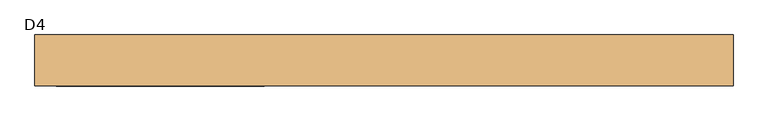
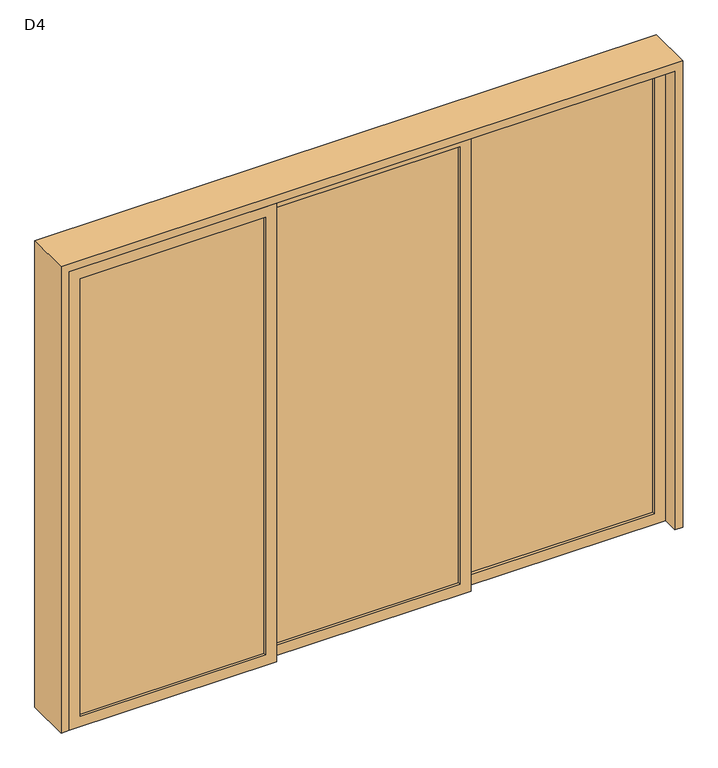
"""IFC4 building model written with IfcOpenShell, lengths in millimetres: door geometry, D4."""

from ifc_helpers import new_model, si_unit, frame, origin, place, context, project, spatial, polyline, outline, extrude, source, transform, mapped, element, save


def d4_ba08b5a2(model_context):
    return source(origin(), model_context, "Body", "SweptSolid", [
        extrude(outline(polyline([(1530.7580012, -5.8333333), (1530.7580012, -19.1666667), (613.2580012, -19.1666667), (613.2580012, -5.8333333), (1530.7580012, -5.8333333)])), frame((0.0, 0.0, 55.0), z_axis=(0.0, 0.0, 1.0), x_axis=(1.0, 0.0, 0.0)), (0.0, 0.0, 1.0), 2290.0),
        extrude(outline(polyline([(0.0, 1585.7580012), (2400.0, 1585.7580012), (2400.0, 558.2580012), (0.0, 558.2580012), (0.0, 1585.7580012)]), holes=[polyline([(55.0, 1530.7580012), (55.0, 613.2580012), (2345.0, 613.2580012), (2345.0, 1530.7580012), (55.0, 1530.7580012)])]), frame((0.0, -32.5, 0.0), z_axis=(0.0, 1.0, 0.0), x_axis=(0.0, 0.0, 1.0)), (0.0, 0.0, 1.0), 40.0),
        extrude(outline(polyline([(544.9246679, -45.8333333), (544.9246679, -59.1666667), (-372.5753321, -59.1666667), (-372.5753321, -45.8333333), (544.9246679, -45.8333333)])), frame((0.0, 0.0, 55.0), z_axis=(0.0, 0.0, 1.0), x_axis=(1.0, 0.0, 0.0)), (0.0, 0.0, 1.0), 2290.0),
        extrude(outline(polyline([(0.0, 599.9246679), (2400.0, 599.9246679), (2400.0, -427.5753321), (0.0, -427.5753321), (0.0, 599.9246679)]), holes=[polyline([(55.0, 544.9246679), (55.0, -372.5753321), (2345.0, -372.5753321), (2345.0, 544.9246679), (55.0, 544.9246679)])]), frame((0.0, -72.5, 0.0), z_axis=(0.0, 1.0, 0.0), x_axis=(0.0, 0.0, 1.0)), (0.0, 0.0, 1.0), 40.0),
        extrude(outline(polyline([(-441.7419988, -85.8333333), (-441.7419988, -99.1666667), (-1359.2419988, -99.1666667), (-1359.2419988, -85.8333333), (-441.7419988, -85.8333333)])), frame((0.0, 0.0, 55.0), z_axis=(0.0, 0.0, 1.0), x_axis=(1.0, 0.0, 0.0)), (0.0, 0.0, 1.0), 2290.0),
        extrude(outline(polyline([(0.0, -386.7419988), (2400.0, -386.7419988), (2400.0, -1414.2419988), (0.0, -1414.2419988), (0.0, -386.7419988)]), holes=[polyline([(55.0, -441.7419988), (55.0, -1359.2419988), (2345.0, -1359.2419988), (2345.0, -441.7419988), (55.0, -441.7419988)])]), frame((0.0, -112.5, 0.0), z_axis=(0.0, 1.0, 0.0), x_axis=(0.0, 0.0, 1.0)), (0.0, 0.0, 1.0), 40.0),
        extrude(outline(polyline([(0.0, -1454.2419988), (0.0, -1414.2419988), (2400.0, -1414.2419988), (2400.0, 1585.7580012), (0.0, 1585.7580012), (0.0, 1625.7580012), (2440.0, 1625.7580012), (2440.0, -1454.2419988), (0.0, -1454.2419988)])), frame((0.0, -112.5, 0.0), z_axis=(0.0, 1.0, 0.0), x_axis=(0.0, 0.0, 1.0)), (0.0, 0.0, 1.0), 225.0),
    ])


if __name__ == "__main__":
    model = new_model("IFC4")
    model_context = context("Model", 3, world=origin())
    ifc_project = project(units=[si_unit("LENGTHUNIT", "METRE", prefix="MILLI")], contexts=[model_context])
    site = spatial("IfcSite", under=ifc_project)
    building = spatial("IfcBuilding", under=site)
    placement = place(None, origin())
    d4_shape = d4_ba08b5a2(model_context)
    element("IfcDoor", 1, ObjectType="D4", at=placement, inside=building, context=model_context, shape_type="MappedRepresentation", body=[
        mapped(d4_shape, transform((0.0, 0.0, 0.0), x_axis=(1.0, 0.0, 0.0), y_axis=(0.0, 1.0, 0.0), z_axis=(0.0, 0.0, 1.0))),
    ])
    save(model, "model.ifc")

# Revit data of these elements
# Type "D4"
#   Type Mark = "59"
#   Operation = "UserDefined"
#   Width = 3000 mm
#   Thickness = 40 mm
#   Rough Width = 3080 mm
#   Rough Height = 2440 mm
#   Panel Width = 1027.5 mm
#   Panel Frame = 55 mm
#   Height = 2400 mm
#   Frame Depth = 40 mm
#   Glass Material = Sliding Door Glass
#   Frame Material = Sliding Door Frame
#   Function = (empty or 0)
# Element 1 (IfcDoor, "D4")
#   Materials on its faces: "Sliding Door Frame", "Sliding Door Glass"
# Materials
#   "Sliding Door Glass": colour RGB 247 247 247, transparency 0.68
#   "Sliding Door Frame": colour RGB 160 107 8, transparency 0
